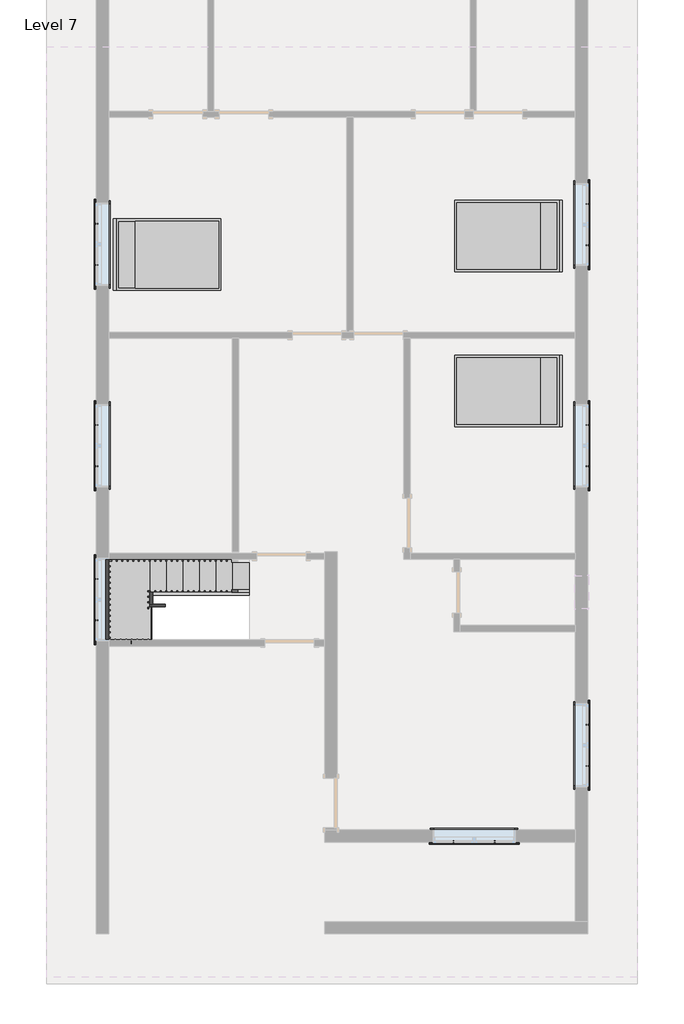
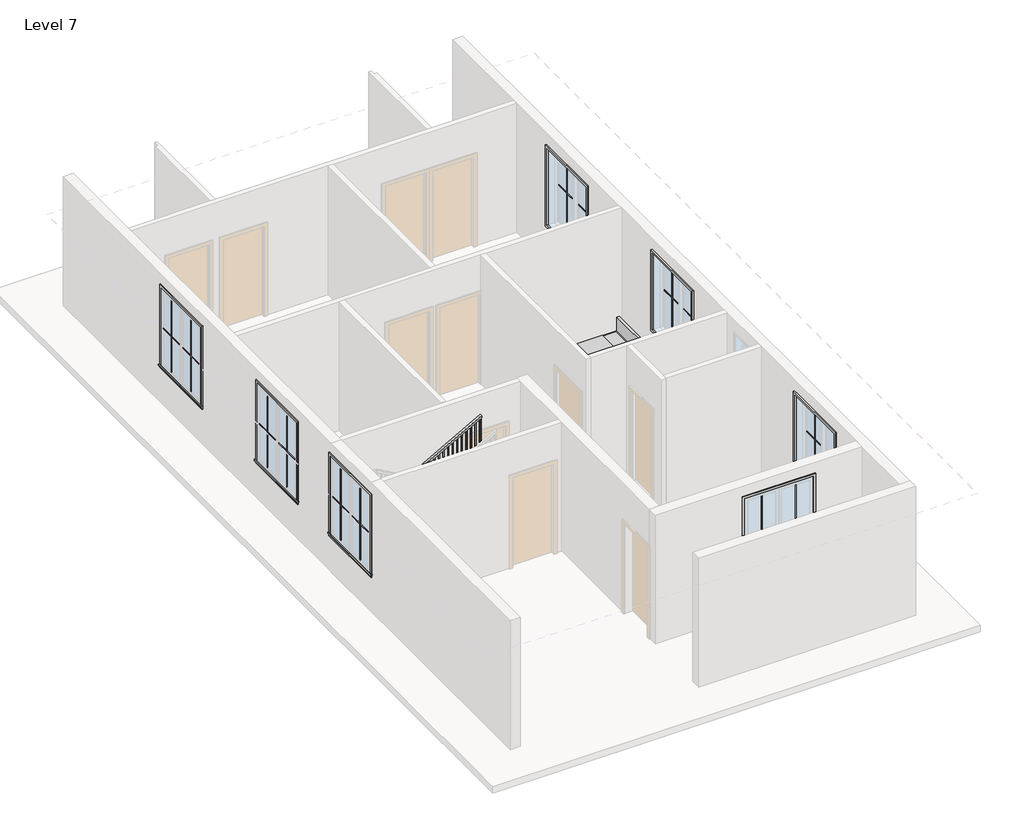
# One storey, part 3 of 3: 28 proxies, 6 members, 3 furniture elements, 1 railing, 1 stair flight.
"""IFC4 building model written with IfcOpenShell, lengths in millimetres."""

from ifc_helpers import new_model, si_unit, frame, origin, place, context, project, spatial, polyline, outline, extrude, faceted_brep, transform, mapped, element, save
from components import muntin_pattern_2x2_muntin_pattern_2x2_f6a80940, muntin_pattern_2x2_muntin_pattern_2x2_09b00a1c, trim_window_exterior_flat_with_sill_698ed857, trim_window_interior_flat_picture_frame_92551a5e, bed_17739_bed_17739_15c61121, stair_flight_6e983af9

model = new_model("IFC4")

# Units and contexts
model_context = context("Model", 3, world=origin())
ifc_project = project(units=[si_unit("LENGTHUNIT", "METRE", prefix="MILLI")], contexts=[model_context])

# Site, building, storey
site = spatial("IfcSite", under=ifc_project)
building = spatial("IfcBuilding", under=site)
storey = spatial("IfcBuildingStorey", under=building, Name="Level 7", Elevation=16002.0)

# Proxies
placement = place(None, origin())
muntin_pattern_2x2_muntin_pattern_2x2_shape = muntin_pattern_2x2_muntin_pattern_2x2_f6a80940(model_context)
element("IfcBuildingElementProxy", 1, Name="Muntin Pattern_2x2 : Muntin Pattern_2x2", ObjectType="Muntin Pattern_2x2 : Muntin Pattern_2x2", at=placement, inside=storey, context=model_context, shape_type="MappedRepresentation", body=[
    mapped(muntin_pattern_2x2_muntin_pattern_2x2_shape, transform((-5778.6870155, 3260.8309309, 16986.25), x_axis=(0.0, 1.0, 0.0), y_axis=(-1.0, 0.0, 0.0), z_axis=(0.0, 0.0, 1.0))),
])
element("IfcBuildingElementProxy", 2, Name="Muntin Pattern_2x2 : Muntin Pattern_2x2", ObjectType="Muntin Pattern_2x2 : Muntin Pattern_2x2", at=placement, inside=storey, context=model_context, shape_type="MappedRepresentation", body=[
    mapped(muntin_pattern_2x2_muntin_pattern_2x2_shape, transform((3270.0629845, 4381.6059309, 16986.25), x_axis=(0.0, -1.0, 0.0), y_axis=(1.0, 0.0, 0.0), z_axis=(0.0, 0.0, 1.0))),
])
element("IfcBuildingElementProxy", 3, Name="Muntin Pattern_2x2 : Muntin Pattern_2x2", ObjectType="Muntin Pattern_2x2 : Muntin Pattern_2x2", at=placement, inside=storey, context=model_context, shape_type="MappedRepresentation", body=[
    mapped(muntin_pattern_2x2_muntin_pattern_2x2_shape, transform((3270.0629845, 304.9059309, 16986.25), x_axis=(0.0, -1.0, 0.0), y_axis=(1.0, 0.0, 0.0), z_axis=(0.0, 0.0, 1.0))),
])
element("IfcBuildingElementProxy", 4, Name="Muntin Pattern_2x2 : Muntin Pattern_2x2", ObjectType="Muntin Pattern_2x2 : Muntin Pattern_2x2", at=placement, inside=storey, context=model_context, shape_type="MappedRepresentation", body=[
    mapped(muntin_pattern_2x2_muntin_pattern_2x2_shape, transform((3270.0629845, -5219.5940691, 16986.25), x_axis=(0.0, -1.0, 0.0), y_axis=(1.0, 0.0, 0.0), z_axis=(0.0, 0.0, 1.0))),
])
element("IfcBuildingElementProxy", 5, Name="Muntin Pattern_2x2 : Muntin Pattern_2x2", ObjectType="Muntin Pattern_2x2 : Muntin Pattern_2x2", at=placement, inside=storey, context=model_context, shape_type="MappedRepresentation", body=[
    mapped(muntin_pattern_2x2_muntin_pattern_2x2_shape, transform((1563.5004845, -7380.1815691, 16986.25), x_axis=(-1.0, 0.0, 0.0), y_axis=(0.0, -1.0, 0.0), z_axis=(0.0, 0.0, 1.0))),
])
element("IfcBuildingElementProxy", 6, Name="Muntin Pattern_2x2 : Muntin Pattern_2x2", ObjectType="Muntin Pattern_2x2 : Muntin Pattern_2x2", at=placement, inside=storey, context=model_context, shape_type="MappedRepresentation", body=[
    mapped(muntin_pattern_2x2_muntin_pattern_2x2_shape, transform((-5778.6870155, -3292.3690691, 16986.25), x_axis=(0.0, 1.0, 0.0), y_axis=(-1.0, 0.0, 0.0), z_axis=(0.0, 0.0, 1.0))),
])
element("IfcBuildingElementProxy", 7, Name="Muntin Pattern_2x2 : Muntin Pattern_2x2", ObjectType="Muntin Pattern_2x2 : Muntin Pattern_2x2", at=placement, inside=storey, context=model_context, shape_type="MappedRepresentation", body=[
    mapped(muntin_pattern_2x2_muntin_pattern_2x2_shape, transform((-5778.6870155, -453.9190691, 16986.25), x_axis=(0.0, 1.0, 0.0), y_axis=(-1.0, 0.0, 0.0), z_axis=(0.0, 0.0, 1.0))),
])
muntin_pattern_2x2_muntin_pattern_2x2_2_shape = muntin_pattern_2x2_muntin_pattern_2x2_09b00a1c(model_context)
element("IfcBuildingElementProxy", 8, Name="Muntin Pattern_2x2 : Muntin Pattern_2x2", ObjectType="Muntin Pattern_2x2 : Muntin Pattern_2x2", at=placement, inside=storey, context=model_context, shape_type="MappedRepresentation", body=[
    mapped(muntin_pattern_2x2_muntin_pattern_2x2_2_shape, transform((-5778.6870155, 4019.6559309, 16986.25), x_axis=(0.0, -1.0, 0.0), y_axis=(1.0, 0.0, 0.0), z_axis=(0.0, 0.0, 1.0))),
])
element("IfcBuildingElementProxy", 9, Name="Muntin Pattern_2x2 : Muntin Pattern_2x2", ObjectType="Muntin Pattern_2x2 : Muntin Pattern_2x2", at=placement, inside=storey, context=model_context, shape_type="MappedRepresentation", body=[
    mapped(muntin_pattern_2x2_muntin_pattern_2x2_2_shape, transform((3270.0629845, 3622.7809309, 16986.25), x_axis=(0.0, 1.0, 0.0), y_axis=(-1.0, 0.0, 0.0), z_axis=(0.0, 0.0, 1.0))),
])
element("IfcBuildingElementProxy", 10, Name="Muntin Pattern_2x2 : Muntin Pattern_2x2", ObjectType="Muntin Pattern_2x2 : Muntin Pattern_2x2", at=placement, inside=storey, context=model_context, shape_type="MappedRepresentation", body=[
    mapped(muntin_pattern_2x2_muntin_pattern_2x2_2_shape, transform((3270.0629845, -453.9190691, 16986.25), x_axis=(0.0, 1.0, 0.0), y_axis=(-1.0, 0.0, 0.0), z_axis=(0.0, 0.0, 1.0))),
])
element("IfcBuildingElementProxy", 11, Name="Muntin Pattern_2x2 : Muntin Pattern_2x2", ObjectType="Muntin Pattern_2x2 : Muntin Pattern_2x2", at=placement, inside=storey, context=model_context, shape_type="MappedRepresentation", body=[
    mapped(muntin_pattern_2x2_muntin_pattern_2x2_2_shape, transform((3270.0629845, -5978.4190691, 16986.25), x_axis=(0.0, 1.0, 0.0), y_axis=(-1.0, 0.0, 0.0), z_axis=(0.0, 0.0, 1.0))),
])
element("IfcBuildingElementProxy", 12, Name="Muntin Pattern_2x2 : Muntin Pattern_2x2", ObjectType="Muntin Pattern_2x2 : Muntin Pattern_2x2", at=placement, inside=storey, context=model_context, shape_type="MappedRepresentation", body=[
    mapped(muntin_pattern_2x2_muntin_pattern_2x2_2_shape, transform((804.6754845, -7380.1815691, 16986.25), x_axis=(1.0, 0.0, 0.0), y_axis=(0.0, 1.0, 0.0), z_axis=(0.0, 0.0, 1.0))),
])
element("IfcBuildingElementProxy", 13, Name="Muntin Pattern_2x2 : Muntin Pattern_2x2", ObjectType="Muntin Pattern_2x2 : Muntin Pattern_2x2", at=placement, inside=storey, context=model_context, shape_type="MappedRepresentation", body=[
    mapped(muntin_pattern_2x2_muntin_pattern_2x2_2_shape, transform((-5778.6870155, -2533.5440691, 16986.25), x_axis=(0.0, -1.0, 0.0), y_axis=(1.0, 0.0, 0.0), z_axis=(0.0, 0.0, 1.0))),
])
element("IfcBuildingElementProxy", 14, Name="Muntin Pattern_2x2 : Muntin Pattern_2x2", ObjectType="Muntin Pattern_2x2 : Muntin Pattern_2x2", at=placement, inside=storey, context=model_context, shape_type="MappedRepresentation", body=[
    mapped(muntin_pattern_2x2_muntin_pattern_2x2_2_shape, transform((-5778.6870155, 304.9059309, 16986.25), x_axis=(0.0, -1.0, 0.0), y_axis=(1.0, 0.0, 0.0), z_axis=(0.0, 0.0, 1.0))),
])
trim_window_exterior_flat_with_sill_shape = trim_window_exterior_flat_with_sill_698ed857(model_context)
element("IfcBuildingElementProxy", 15, Name="Trim-Window-Exterior-Flat : with Sill", ObjectType="Trim-Window-Exterior-Flat : with Sill", at=placement, inside=storey, context=model_context, shape_type="MappedRepresentation", body=[
    mapped(trim_window_exterior_flat_with_sill_shape, transform((-5788.2120155, 3640.2434309, 18745.2), x_axis=(0.0, -1.0, 0.0), y_axis=(0.0, 0.0, 1.0), z_axis=(-1.0, 0.0, 0.0))),
])
element("IfcBuildingElementProxy", 16, Name="Trim-Window-Exterior-Flat : with Sill", ObjectType="Trim-Window-Exterior-Flat : with Sill", at=placement, inside=storey, context=model_context, shape_type="MappedRepresentation", body=[
    mapped(trim_window_exterior_flat_with_sill_shape, transform((3279.5879845, 4002.1934309, 18745.2), x_axis=(0.0, 1.0, 0.0), y_axis=(0.0, 0.0, 1.0), z_axis=(1.0, 0.0, 0.0))),
])
element("IfcBuildingElementProxy", 17, Name="Trim-Window-Exterior-Flat : with Sill", ObjectType="Trim-Window-Exterior-Flat : with Sill", at=placement, inside=storey, context=model_context, shape_type="MappedRepresentation", body=[
    mapped(trim_window_exterior_flat_with_sill_shape, transform((3279.5879845, -74.5065691, 18745.2), x_axis=(0.0, 1.0, 0.0), y_axis=(0.0, 0.0, 1.0), z_axis=(1.0, 0.0, 0.0))),
])
element("IfcBuildingElementProxy", 18, Name="Trim-Window-Exterior-Flat : with Sill", ObjectType="Trim-Window-Exterior-Flat : with Sill", at=placement, inside=storey, context=model_context, shape_type="MappedRepresentation", body=[
    mapped(trim_window_exterior_flat_with_sill_shape, transform((3279.5879845, -5599.0065691, 18745.2), x_axis=(0.0, 1.0, 0.0), y_axis=(0.0, 0.0, 1.0), z_axis=(1.0, 0.0, 0.0))),
])
element("IfcBuildingElementProxy", 19, Name="Trim-Window-Exterior-Flat : with Sill", ObjectType="Trim-Window-Exterior-Flat : with Sill", at=placement, inside=storey, context=model_context, shape_type="MappedRepresentation", body=[
    mapped(trim_window_exterior_flat_with_sill_shape, transform((1184.0879845, -7389.7065691, 18745.2), x_axis=(1.0, 0.0, 0.0), y_axis=(0.0, 0.0, 1.0), z_axis=(0.0, -1.0, 0.0))),
])
element("IfcBuildingElementProxy", 20, Name="Trim-Window-Exterior-Flat : with Sill", ObjectType="Trim-Window-Exterior-Flat : with Sill", at=placement, inside=storey, context=model_context, shape_type="MappedRepresentation", body=[
    mapped(trim_window_exterior_flat_with_sill_shape, transform((-5788.2120155, -2912.9565691, 18745.2), x_axis=(0.0, -1.0, 0.0), y_axis=(0.0, 0.0, 1.0), z_axis=(-1.0, 0.0, 0.0))),
])
element("IfcBuildingElementProxy", 21, Name="Trim-Window-Exterior-Flat : with Sill", ObjectType="Trim-Window-Exterior-Flat : with Sill", at=placement, inside=storey, context=model_context, shape_type="MappedRepresentation", body=[
    mapped(trim_window_exterior_flat_with_sill_shape, transform((-5788.2120155, -74.5065691, 18745.2), x_axis=(0.0, -1.0, 0.0), y_axis=(0.0, 0.0, 1.0), z_axis=(-1.0, 0.0, 0.0))),
])
trim_window_interior_flat_picture_frame_shape = trim_window_interior_flat_picture_frame_92551a5e(model_context)
element("IfcBuildingElementProxy", 22, Name="Trim-Window-Interior-Flat : Picture Frame", ObjectType="Trim-Window-Interior-Flat : Picture Frame", at=placement, inside=storey, context=model_context, shape_type="MappedRepresentation", body=[
    mapped(trim_window_interior_flat_picture_frame_shape, transform((-5559.6120155, 3640.2434309, 18745.2), x_axis=(0.0, 1.0, 0.0), y_axis=(0.0, 0.0, 1.0), z_axis=(1.0, 0.0, 0.0))),
])
element("IfcBuildingElementProxy", 23, Name="Trim-Window-Interior-Flat : Picture Frame", ObjectType="Trim-Window-Interior-Flat : Picture Frame", at=placement, inside=storey, context=model_context, shape_type="MappedRepresentation", body=[
    mapped(trim_window_interior_flat_picture_frame_shape, transform((3050.9879845, 4002.1934309, 18745.2), x_axis=(0.0, -1.0, 0.0), y_axis=(0.0, 0.0, 1.0), z_axis=(-1.0, 0.0, 0.0))),
])
element("IfcBuildingElementProxy", 24, Name="Trim-Window-Interior-Flat : Picture Frame", ObjectType="Trim-Window-Interior-Flat : Picture Frame", at=placement, inside=storey, context=model_context, shape_type="MappedRepresentation", body=[
    mapped(trim_window_interior_flat_picture_frame_shape, transform((3050.9879845, -74.5065691, 18745.2), x_axis=(0.0, -1.0, 0.0), y_axis=(0.0, 0.0, 1.0), z_axis=(-1.0, 0.0, 0.0))),
])
element("IfcBuildingElementProxy", 25, Name="Trim-Window-Interior-Flat : Picture Frame", ObjectType="Trim-Window-Interior-Flat : Picture Frame", at=placement, inside=storey, context=model_context, shape_type="MappedRepresentation", body=[
    mapped(trim_window_interior_flat_picture_frame_shape, transform((3050.9879845, -5599.0065691, 18745.2), x_axis=(0.0, -1.0, 0.0), y_axis=(0.0, 0.0, 1.0), z_axis=(-1.0, 0.0, 0.0))),
])
element("IfcBuildingElementProxy", 26, Name="Trim-Window-Interior-Flat : Picture Frame", ObjectType="Trim-Window-Interior-Flat : Picture Frame", at=placement, inside=storey, context=model_context, shape_type="MappedRepresentation", body=[
    mapped(trim_window_interior_flat_picture_frame_shape, transform((1184.0879845, -7161.1065691, 18745.2), x_axis=(-1.0, 0.0, 0.0), y_axis=(0.0, 0.0, 1.0), z_axis=(0.0, 1.0, 0.0))),
])
element("IfcBuildingElementProxy", 27, Name="Trim-Window-Interior-Flat : Picture Frame", ObjectType="Trim-Window-Interior-Flat : Picture Frame", at=placement, inside=storey, context=model_context, shape_type="MappedRepresentation", body=[
    mapped(trim_window_interior_flat_picture_frame_shape, transform((-5559.6120155, -2912.9565691, 18745.2), x_axis=(0.0, 1.0, 0.0), y_axis=(0.0, 0.0, 1.0), z_axis=(1.0, 0.0, 0.0))),
])
element("IfcBuildingElementProxy", 28, Name="Trim-Window-Interior-Flat : Picture Frame", ObjectType="Trim-Window-Interior-Flat : Picture Frame", at=placement, inside=storey, context=model_context, shape_type="MappedRepresentation", body=[
    mapped(trim_window_interior_flat_picture_frame_shape, transform((-5559.6120155, -74.5065691, 18745.2), x_axis=(0.0, 1.0, 0.0), y_axis=(0.0, 0.0, 1.0), z_axis=(1.0, 0.0, 0.0))),
])

# Furniture
bed_17739_bed_17739_shape = bed_17739_bed_17739_15c61121(model_context)
element("IfcFurniture", 29, ObjectType="Bed_17739 : Bed_17739", at=placement, inside=storey, context=model_context, shape_type="MappedRepresentation", body=[
    mapped(bed_17739_bed_17739_shape, transform((-4454.7120155, 3449.7434309, 16002.0), x_axis=(0.0, 1.0, 0.0), y_axis=(-1.0, 0.0, 0.0), z_axis=(0.0, 0.0, 1.0))),
])
element("IfcFurniture", 30, ObjectType="Bed_17739 : Bed_17739", at=placement, inside=storey, context=model_context, shape_type="MappedRepresentation", body=[
    mapped(bed_17739_bed_17739_shape, transform((1793.6879845, 3792.6434309, 16002.0), x_axis=(0.0, -1.0, 0.0), y_axis=(1.0, 0.0, 0.0), z_axis=(0.0, 0.0, 1.0))),
])
element("IfcFurniture", 31, ObjectType="Bed_17739 : Bed_17739", at=placement, inside=storey, context=model_context, shape_type="MappedRepresentation", body=[
    mapped(bed_17739_bed_17739_shape, transform((1793.6879845, 935.1434309, 16002.0), x_axis=(0.0, -1.0, 0.0), y_axis=(1.0, 0.0, 0.0), z_axis=(0.0, 0.0, 1.0))),
])

# Members
element("IfcMember", 32, ObjectType="Stringer - 2\" Width", at=placement, inside=storey, context=model_context, shape_type="SweptSolid", body=[
    extrude(outline(polyline([(16002.0, -2968.8120155), (16209.5983948, -2968.8120155), (17197.3761726, -4746.8120155), (16848.6974984, -4746.8120155), (16002.0, -3222.7565183), (16002.0, -2968.8120155)])), frame((0.0, -2830.4065691, 0.0), z_axis=(0.0, 1.0, 0.0), x_axis=(0.0, 0.0, 1.0)), (0.0, 0.0, 1.0), 50.8),
])
element("IfcMember", 33, ObjectType="Stringer - 2\" Width", at=placement, inside=storey, context=model_context, shape_type="SweptSolid", body=[
    extrude(outline(polyline([(-4797.6120155, -2779.6065691), (-4746.8120155, -2779.6065691), (-4746.8120155, -2995.5065691), (-4797.6120155, -2995.5065691), (-4797.6120155, -2779.6065691)])), frame((0.0, 0.0, 16958.7333333), z_axis=(0.0, 0.0, 1.0), x_axis=(1.0, 0.0, 0.0)), (0.0, 0.0, 1.0), 304.8),
])
element("IfcMember", 34, ObjectType="Stringer - 2\" Width", at=placement, inside=storey, context=model_context, shape_type="SweptSolid", body=[
    extrude(outline(polyline([(17394.9317281, -4797.6120155), (17046.253054, -4797.6120155), (18062.253054, -2968.8120155), (18410.9317281, -2968.8120155), (17394.9317281, -4797.6120155)])), frame((0.0, -3046.3065691, 0.0), z_axis=(0.0, 1.0, 0.0), x_axis=(0.0, 0.0, 1.0)), (0.0, 0.0, 1.0), 50.8),
])
element("IfcMember", 35, ObjectType="Stringer - 2\" Width", at=placement, inside=storey, context=model_context, shape_type="SweptSolid", body=[
    extrude(outline(polyline([(16002.0, -2968.8120155), (16209.5983948, -2968.8120155), (17263.5333333, -4865.8949049), (17263.5333333, -5493.5165183), (16002.0, -3222.7565183), (16002.0, -2968.8120155)])), frame((0.0, -2170.0065691, 0.0), z_axis=(0.0, 1.0, 0.0), x_axis=(0.0, 0.0, 1.0)), (0.0, 0.0, 1.0), 50.8),
])
element("IfcMember", 36, ObjectType="Stringer - 2\" Width", at=placement, inside=storey, context=model_context, shape_type="SweptSolid", body=[
    extrude(outline(polyline([(-5610.4120155, -2119.2065691), (-5559.6120155, -2119.2065691), (-5559.6120155, -3674.9565691), (-5610.4120155, -3674.9565691), (-5610.4120155, -2119.2065691)])), frame((0.0, 0.0, 16958.7333333), z_axis=(0.0, 0.0, 1.0), x_axis=(1.0, 0.0, 0.0)), (0.0, 0.0, 1.0), 304.8),
])
element("IfcMember", 37, ObjectType="Stringer - 2\" Width", at=placement, inside=storey, context=model_context, shape_type="SweptSolid", body=[
    extrude(outline(polyline([(16958.7333333, -4955.1475127), (18062.253054, -2968.8120155), (18410.9317281, -2968.8120155), (16958.7333333, -5582.7691261), (16958.7333333, -4955.1475127)])), frame((0.0, -3725.7565691, 0.0), z_axis=(0.0, 1.0, 0.0), x_axis=(0.0, 0.0, 1.0)), (0.0, 0.0, 1.0), 50.8),
])

# Railing
element("IfcRailing", 38, ObjectType="Handrail - Rectangular", at=placement, inside=storey, context=model_context, shape_type="SolidModel", body=[
    faceted_brep([(-2968.8120155, -2779.6065691, 17085.7333333), (-2968.8120155, -2779.6065691, 17027.620221), (-2968.8120155, -2728.8065691, 17027.620221), (-2968.8120155, -2728.8065691, 17085.7333333), (-4721.4120155, -2779.6065691, 18059.4), (-4772.2120155, -2779.6065691, 18029.5091099), (-4772.2120155, -2728.8065691, 18029.5091099), (-4721.4120155, -2728.8065691, 18059.4), (-4721.4120155, -2779.6065691, 18101.7333333), (-4772.2120155, -2779.6065691, 18050.9333333), (-4772.2120155, -2728.8065691, 18050.9333333), (-4721.4120155, -2728.8065691, 18101.7333333), (-4797.6120155, -2779.6065691, 18101.7333333), (-4797.6120155, -2779.6065691, 18050.9333333), (-4848.4120155, -2728.8065691, 18050.9333333), (-4848.4120155, -2728.8065691, 18101.7333333), (-4797.6120155, -2855.8065691, 18101.7333333), (-4797.6120155, -2855.8065691, 18050.9333333), (-4848.4120155, -2855.8065691, 18050.9333333), (-4848.4120155, -2855.8065691, 18101.7333333), (-4797.6120155, -2970.1065691, 18101.7333333), (-4797.6120155, -3020.9065691, 18050.9333333), (-4848.4120155, -3020.9065691, 18050.9333333), (-4848.4120155, -2970.1065691, 18101.7333333), (-4797.6120155, -2970.1065691, 18313.4), (-4797.6120155, -3020.9065691, 18262.6), (-4848.4120155, -3020.9065691, 18262.6), (-4848.4120155, -2970.1065691, 18313.4), (-4797.6120155, -3046.3065691, 18313.4), (-4797.6120155, -3046.3065691, 18262.6), (-4848.4120155, -3097.1065691, 18262.6), (-4848.4120155, -3097.1065691, 18313.4), (-4721.4120155, -3046.3065691, 18313.4), (-4708.2484132, -3046.3065691, 18262.6), (-4708.2484132, -3097.1065691, 18262.6), (-4721.4120155, -3097.1065691, 18313.4), (-2968.8120155, -3046.3065691, 19287.0666667), (-2968.8120155, -3097.1065691, 19287.0666667), (-2968.8120155, -3097.1065691, 19228.9535543), (-2968.8120155, -3046.3065691, 19228.9535543)], [[[0, 1, 2, 3]], [[1, 0, 4, 5]], [[2, 1, 5, 6]], [[3, 2, 6, 7]], [[0, 3, 7, 4]], [[5, 4, 8, 9]], [[6, 5, 9, 10]], [[7, 6, 10, 11]], [[4, 7, 11, 8]], [[9, 8, 12, 13]], [[10, 9, 13, 14]], [[11, 10, 14, 15]], [[8, 11, 15, 12]], [[13, 12, 16, 17]], [[14, 13, 17, 18]], [[15, 14, 18, 19]], [[12, 15, 19, 16]], [[17, 16, 20, 21]], [[18, 17, 21, 22]], [[19, 18, 22, 23]], [[16, 19, 23, 20]], [[21, 20, 24, 25]], [[22, 21, 25, 26]], [[23, 22, 26, 27]], [[20, 23, 27, 24]], [[25, 24, 28, 29]], [[26, 25, 29, 30]], [[27, 26, 30, 31]], [[24, 27, 31, 28]], [[29, 28, 32, 33]], [[30, 29, 33, 34]], [[31, 30, 34, 35]], [[28, 31, 35, 32]], [[36, 37, 38, 39]], [[33, 32, 36, 39]], [[34, 33, 39, 38]], [[35, 34, 38, 37]], [[32, 35, 37, 36]]]),
    extrude(outline(polyline([(19209.5507765, -3003.7370155), (18203.3333333, -3003.7370155), (18203.3333333, -2984.6870155), (19220.1341099, -2984.6870155), (19209.5507765, -3003.7370155)])), frame((0.0, -3081.2315691, 0.0), z_axis=(0.0, 1.0, 0.0), x_axis=(0.0, 0.0, 1.0)), (0.0, 0.0, 1.0), 19.05),
    extrude(outline(polyline([(19153.1063321, -3105.3370155), (18203.3333333, -3105.3370155), (18203.3333333, -3086.2870155), (19163.6896654, -3086.2870155), (19153.1063321, -3105.3370155)])), frame((0.0, -3081.2315691, 0.0), z_axis=(0.0, 1.0, 0.0), x_axis=(0.0, 0.0, 1.0)), (0.0, 0.0, 1.0), 19.05),
    extrude(outline(polyline([(19096.6618876, -3206.9370155), (18203.3333333, -3206.9370155), (18203.3333333, -3187.8870155), (19107.245221, -3187.8870155), (19096.6618876, -3206.9370155)])), frame((0.0, -3081.2315691, 0.0), z_axis=(0.0, 1.0, 0.0), x_axis=(0.0, 0.0, 1.0)), (0.0, 0.0, 1.0), 19.05),
    extrude(outline(polyline([(19040.2174432, -3308.5370155), (18034.0, -3308.5370155), (18034.0, -3289.4870155), (19050.8007765, -3289.4870155), (19040.2174432, -3308.5370155)])), frame((0.0, -3081.2315691, 0.0), z_axis=(0.0, 1.0, 0.0), x_axis=(0.0, 0.0, 1.0)), (0.0, 0.0, 1.0), 19.05),
    extrude(outline(polyline([(18983.7729988, -3410.1370155), (18034.0, -3410.1370155), (18034.0, -3391.0870155), (18994.3563321, -3391.0870155), (18983.7729988, -3410.1370155)])), frame((0.0, -3081.2315691, 0.0), z_axis=(0.0, 1.0, 0.0), x_axis=(0.0, 0.0, 1.0)), (0.0, 0.0, 1.0), 19.05),
    extrude(outline(polyline([(18927.3285543, -3511.7370155), (18034.0, -3511.7370155), (18034.0, -3492.6870155), (18937.9118876, -3492.6870155), (18927.3285543, -3511.7370155)])), frame((0.0, -3081.2315691, 0.0), z_axis=(0.0, 1.0, 0.0), x_axis=(0.0, 0.0, 1.0)), (0.0, 0.0, 1.0), 19.05),
    extrude(outline(polyline([(18870.8841099, -3613.3370155), (17864.6666667, -3613.3370155), (17864.6666667, -3594.2870155), (18881.4674432, -3594.2870155), (18870.8841099, -3613.3370155)])), frame((0.0, -3081.2315691, 0.0), z_axis=(0.0, 1.0, 0.0), x_axis=(0.0, 0.0, 1.0)), (0.0, 0.0, 1.0), 19.05),
    extrude(outline(polyline([(18814.4396654, -3714.9370155), (17864.6666667, -3714.9370155), (17864.6666667, -3695.8870155), (18825.0229988, -3695.8870155), (18814.4396654, -3714.9370155)])), frame((0.0, -3081.2315691, 0.0), z_axis=(0.0, 1.0, 0.0), x_axis=(0.0, 0.0, 1.0)), (0.0, 0.0, 1.0), 19.05),
    extrude(outline(polyline([(18757.995221, -3816.5370155), (17864.6666667, -3816.5370155), (17864.6666667, -3797.4870155), (18768.5785543, -3797.4870155), (18757.995221, -3816.5370155)])), frame((0.0, -3081.2315691, 0.0), z_axis=(0.0, 1.0, 0.0), x_axis=(0.0, 0.0, 1.0)), (0.0, 0.0, 1.0), 19.05),
    extrude(outline(polyline([(18701.5507765, -3918.1370155), (17695.3333333, -3918.1370155), (17695.3333333, -3899.0870155), (18712.1341099, -3899.0870155), (18701.5507765, -3918.1370155)])), frame((0.0, -3081.2315691, 0.0), z_axis=(0.0, 1.0, 0.0), x_axis=(0.0, 0.0, 1.0)), (0.0, 0.0, 1.0), 19.05),
    extrude(outline(polyline([(18645.1063321, -4019.7370155), (17695.3333333, -4019.7370155), (17695.3333333, -4000.6870155), (18655.6896654, -4000.6870155), (18645.1063321, -4019.7370155)])), frame((0.0, -3081.2315691, 0.0), z_axis=(0.0, 1.0, 0.0), x_axis=(0.0, 0.0, 1.0)), (0.0, 0.0, 1.0), 19.05),
    extrude(outline(polyline([(18588.6618876, -4121.3370155), (17695.3333333, -4121.3370155), (17695.3333333, -4102.2870155), (18599.245221, -4102.2870155), (18588.6618876, -4121.3370155)])), frame((0.0, -3081.2315691, 0.0), z_axis=(0.0, 1.0, 0.0), x_axis=(0.0, 0.0, 1.0)), (0.0, 0.0, 1.0), 19.05),
    extrude(outline(polyline([(18532.2174432, -4222.9370155), (17526.0, -4222.9370155), (17526.0, -4203.8870155), (18542.8007765, -4203.8870155), (18532.2174432, -4222.9370155)])), frame((0.0, -3081.2315691, 0.0), z_axis=(0.0, 1.0, 0.0), x_axis=(0.0, 0.0, 1.0)), (0.0, 0.0, 1.0), 19.05),
    extrude(outline(polyline([(18475.7729988, -4324.5370155), (17526.0, -4324.5370155), (17526.0, -4305.4870155), (18486.3563321, -4305.4870155), (18475.7729988, -4324.5370155)])), frame((0.0, -3081.2315691, 0.0), z_axis=(0.0, 1.0, 0.0), x_axis=(0.0, 0.0, 1.0)), (0.0, 0.0, 1.0), 19.05),
    extrude(outline(polyline([(18419.3285543, -4426.1370155), (17526.0, -4426.1370155), (17526.0, -4407.0870155), (18429.9118876, -4407.0870155), (18419.3285543, -4426.1370155)])), frame((0.0, -3081.2315691, 0.0), z_axis=(0.0, 1.0, 0.0), x_axis=(0.0, 0.0, 1.0)), (0.0, 0.0, 1.0), 19.05),
    extrude(outline(polyline([(18362.8841099, -4527.7370155), (17356.6666667, -4527.7370155), (17356.6666667, -4508.6870155), (18373.4674432, -4508.6870155), (18362.8841099, -4527.7370155)])), frame((0.0, -3081.2315691, 0.0), z_axis=(0.0, 1.0, 0.0), x_axis=(0.0, 0.0, 1.0)), (0.0, 0.0, 1.0), 19.05),
    extrude(outline(polyline([(18306.4396654, -4629.3370155), (17356.6666667, -4629.3370155), (17356.6666667, -4610.2870155), (18317.0229988, -4610.2870155), (18306.4396654, -4629.3370155)])), frame((0.0, -3081.2315691, 0.0), z_axis=(0.0, 1.0, 0.0), x_axis=(0.0, 0.0, 1.0)), (0.0, 0.0, 1.0), 19.05),
    extrude(outline(polyline([(18249.995221, -4730.9370155), (17356.6666667, -4730.9370155), (17356.6666667, -4711.8870155), (18260.5785543, -4711.8870155), (18249.995221, -4730.9370155)])), frame((0.0, -3081.2315691, 0.0), z_axis=(0.0, 1.0, 0.0), x_axis=(0.0, 0.0, 1.0)), (0.0, 0.0, 1.0), 19.05),
    extrude(outline(polyline([(-4813.4870155, -3049.4815691), (-4813.4870155, -3068.5315691), (-4832.5370155, -3068.5315691), (-4832.5370155, -3049.4815691), (-4813.4870155, -3049.4815691)])), frame((0.0, 0.0, 17187.3333333), z_axis=(0.0, 0.0, 1.0), x_axis=(1.0, 0.0, 0.0)), (0.0, 0.0, 1.0), 1075.2666667),
    extrude(outline(polyline([(-4813.4870155, -2947.8815691), (-4813.4870155, -2966.9315691), (-4832.5370155, -2966.9315691), (-4832.5370155, -2947.8815691), (-4813.4870155, -2947.8815691)])), frame((0.0, 0.0, 17187.3333333), z_axis=(0.0, 0.0, 1.0), x_axis=(1.0, 0.0, 0.0)), (0.0, 0.0, 1.0), 863.6),
    extrude(outline(polyline([(-4813.4870155, -2846.2815691), (-4813.4870155, -2865.3315691), (-4832.5370155, -2865.3315691), (-4832.5370155, -2846.2815691), (-4813.4870155, -2846.2815691)])), frame((0.0, 0.0, 17187.3333333), z_axis=(0.0, 0.0, 1.0), x_axis=(1.0, 0.0, 0.0)), (0.0, 0.0, 1.0), 863.6),
    extrude(outline(polyline([(-4788.0870155, -2763.7315691), (-4807.1370155, -2763.7315691), (-4807.1370155, -2744.6815691), (-4788.0870155, -2744.6815691), (-4788.0870155, -2763.7315691)])), frame((0.0, 0.0, 17187.3333333), z_axis=(0.0, 0.0, 1.0), x_axis=(1.0, 0.0, 0.0)), (0.0, 0.0, 1.0), 863.6),
    extrude(outline(polyline([(17992.4674432, -4705.5370155), (17018.0, -4705.5370155), (17018.0, -4686.4870155), (17981.8841099, -4686.4870155), (17992.4674432, -4705.5370155)])), frame((0.0, -2763.7315691, 0.0), z_axis=(0.0, 1.0, 0.0), x_axis=(0.0, 0.0, 1.0)), (0.0, 0.0, 1.0), 19.05),
    extrude(outline(polyline([(17936.0229988, -4603.9370155), (17018.0, -4603.9370155), (17018.0, -4584.8870155), (17925.4396654, -4584.8870155), (17936.0229988, -4603.9370155)])), frame((0.0, -2763.7315691, 0.0), z_axis=(0.0, 1.0, 0.0), x_axis=(0.0, 0.0, 1.0)), (0.0, 0.0, 1.0), 19.05),
    extrude(outline(polyline([(17879.5785543, -4502.3370155), (17018.0, -4502.3370155), (17018.0, -4483.2870155), (17868.995221, -4483.2870155), (17879.5785543, -4502.3370155)])), frame((0.0, -2763.7315691, 0.0), z_axis=(0.0, 1.0, 0.0), x_axis=(0.0, 0.0, 1.0)), (0.0, 0.0, 1.0), 19.05),
    extrude(outline(polyline([(17823.1341099, -4400.7370155), (16848.6666667, -4400.7370155), (16848.6666667, -4381.6870155), (17812.5507765, -4381.6870155), (17823.1341099, -4400.7370155)])), frame((0.0, -2763.7315691, 0.0), z_axis=(0.0, 1.0, 0.0), x_axis=(0.0, 0.0, 1.0)), (0.0, 0.0, 1.0), 19.05),
    extrude(outline(polyline([(17766.6896654, -4299.1370155), (16848.6666667, -4299.1370155), (16848.6666667, -4280.0870155), (17756.1063321, -4280.0870155), (17766.6896654, -4299.1370155)])), frame((0.0, -2763.7315691, 0.0), z_axis=(0.0, 1.0, 0.0), x_axis=(0.0, 0.0, 1.0)), (0.0, 0.0, 1.0), 19.05),
    extrude(outline(polyline([(17710.245221, -4197.5370155), (16848.6666667, -4197.5370155), (16848.6666667, -4178.4870155), (17699.6618876, -4178.4870155), (17710.245221, -4197.5370155)])), frame((0.0, -2763.7315691, 0.0), z_axis=(0.0, 1.0, 0.0), x_axis=(0.0, 0.0, 1.0)), (0.0, 0.0, 1.0), 19.05),
    extrude(outline(polyline([(17653.8007765, -4095.9370155), (16679.3333333, -4095.9370155), (16679.3333333, -4076.8870155), (17643.2174432, -4076.8870155), (17653.8007765, -4095.9370155)])), frame((0.0, -2763.7315691, 0.0), z_axis=(0.0, 1.0, 0.0), x_axis=(0.0, 0.0, 1.0)), (0.0, 0.0, 1.0), 19.05),
    extrude(outline(polyline([(17597.3563321, -3994.3370155), (16679.3333333, -3994.3370155), (16679.3333333, -3975.2870155), (17586.7729988, -3975.2870155), (17597.3563321, -3994.3370155)])), frame((0.0, -2763.7315691, 0.0), z_axis=(0.0, 1.0, 0.0), x_axis=(0.0, 0.0, 1.0)), (0.0, 0.0, 1.0), 19.05),
    extrude(outline(polyline([(17540.9118876, -3892.7370155), (16679.3333333, -3892.7370155), (16679.3333333, -3873.6870155), (17530.3285543, -3873.6870155), (17540.9118876, -3892.7370155)])), frame((0.0, -2763.7315691, 0.0), z_axis=(0.0, 1.0, 0.0), x_axis=(0.0, 0.0, 1.0)), (0.0, 0.0, 1.0), 19.05),
    extrude(outline(polyline([(17484.4674432, -3791.1370155), (16510.0, -3791.1370155), (16510.0, -3772.0870155), (17473.8841099, -3772.0870155), (17484.4674432, -3791.1370155)])), frame((0.0, -2763.7315691, 0.0), z_axis=(0.0, 1.0, 0.0), x_axis=(0.0, 0.0, 1.0)), (0.0, 0.0, 1.0), 19.05),
    extrude(outline(polyline([(17428.0229988, -3689.5370155), (16510.0, -3689.5370155), (16510.0, -3670.4870155), (17417.4396654, -3670.4870155), (17428.0229988, -3689.5370155)])), frame((0.0, -2763.7315691, 0.0), z_axis=(0.0, 1.0, 0.0), x_axis=(0.0, 0.0, 1.0)), (0.0, 0.0, 1.0), 19.05),
    extrude(outline(polyline([(17371.5785543, -3587.9370155), (16510.0, -3587.9370155), (16510.0, -3568.8870155), (17360.995221, -3568.8870155), (17371.5785543, -3587.9370155)])), frame((0.0, -2763.7315691, 0.0), z_axis=(0.0, 1.0, 0.0), x_axis=(0.0, 0.0, 1.0)), (0.0, 0.0, 1.0), 19.05),
    extrude(outline(polyline([(17315.1341099, -3486.3370155), (16340.6666667, -3486.3370155), (16340.6666667, -3467.2870155), (17304.5507765, -3467.2870155), (17315.1341099, -3486.3370155)])), frame((0.0, -2763.7315691, 0.0), z_axis=(0.0, 1.0, 0.0), x_axis=(0.0, 0.0, 1.0)), (0.0, 0.0, 1.0), 19.05),
    extrude(outline(polyline([(17258.6896654, -3384.7370155), (16340.6666667, -3384.7370155), (16340.6666667, -3365.6870155), (17248.1063321, -3365.6870155), (17258.6896654, -3384.7370155)])), frame((0.0, -2763.7315691, 0.0), z_axis=(0.0, 1.0, 0.0), x_axis=(0.0, 0.0, 1.0)), (0.0, 0.0, 1.0), 19.05),
    extrude(outline(polyline([(17202.245221, -3283.1370155), (16340.6666667, -3283.1370155), (16340.6666667, -3264.0870155), (17191.6618876, -3264.0870155), (17202.245221, -3283.1370155)])), frame((0.0, -2763.7315691, 0.0), z_axis=(0.0, 1.0, 0.0), x_axis=(0.0, 0.0, 1.0)), (0.0, 0.0, 1.0), 19.05),
    extrude(outline(polyline([(17145.8007765, -3181.5370155), (16171.3333333, -3181.5370155), (16171.3333333, -3162.4870155), (17135.2174432, -3162.4870155), (17145.8007765, -3181.5370155)])), frame((0.0, -2763.7315691, 0.0), z_axis=(0.0, 1.0, 0.0), x_axis=(0.0, 0.0, 1.0)), (0.0, 0.0, 1.0), 19.05),
    extrude(outline(polyline([(17089.3563321, -3079.9370155), (16171.3333333, -3079.9370155), (16171.3333333, -3060.8870155), (17078.7729988, -3060.8870155), (17089.3563321, -3079.9370155)])), frame((0.0, -2763.7315691, 0.0), z_axis=(0.0, 1.0, 0.0), x_axis=(0.0, 0.0, 1.0)), (0.0, 0.0, 1.0), 19.05),
    extrude(outline(polyline([(-4813.4870155, -3062.1815691), (-4813.4870155, -3081.2315691), (-4832.5370155, -3081.2315691), (-4832.5370155, -3062.1815691), (-4813.4870155, -3062.1815691)])), frame((0.0, 0.0, 17187.3333333), z_axis=(0.0, 0.0, 1.0), x_axis=(1.0, 0.0, 0.0)), (0.0, 0.0, 1.0), 1075.2666667),
    extrude(outline(polyline([(-4813.4870155, -2763.7315691), (-4832.5370155, -2763.7315691), (-4832.5370155, -2744.6815691), (-4813.4870155, -2744.6815691), (-4813.4870155, -2763.7315691)])), frame((0.0, 0.0, 17187.3333333), z_axis=(0.0, 0.0, 1.0), x_axis=(1.0, 0.0, 0.0)), (0.0, 0.0, 1.0), 863.6),
    extrude(outline(polyline([(19218.370221, -2987.8620155), (18203.3333333, -2987.8620155), (18203.3333333, -2968.8120155), (19228.9535543, -2968.8120155), (19218.370221, -2987.8620155)])), frame((0.0, -3081.2315691, 0.0), z_axis=(0.0, 1.0, 0.0), x_axis=(0.0, 0.0, 1.0)), (0.0, 0.0, 1.0), 19.05),
    extrude(outline(polyline([(17038.2035543, -2987.8620155), (16171.3333333, -2987.8620155), (16171.3333333, -2968.8120155), (17027.620221, -2968.8120155), (17038.2035543, -2987.8620155)])), frame((0.0, -2763.7315691, 0.0), z_axis=(0.0, 1.0, 0.0), x_axis=(0.0, 0.0, 1.0)), (0.0, 0.0, 1.0), 19.05),
])

# Stair flight
stair_flight_shape = stair_flight_6e983af9(model_context)
element("IfcStairFlight", 39, ObjectType="2\" Tread 1\" Nosing 1/4\" Riser", at=placement, inside=storey, context=model_context, shape_type="MappedRepresentation", body=[
    mapped(stair_flight_shape, transform((0.0, 0.0, 0.0), x_axis=(1.0, 0.0, 0.0), y_axis=(0.0, 1.0, 0.0), z_axis=(0.0, 0.0, 1.0))),
])

save(model, "model.ifc")

# Revit data of these elements
# Type "Muntin Pattern_2x2 : Muntin Pattern_2x2"
#   Width [instance default] = 4' - 0"
#   Thickness = 0' - 0 1/2"
#   Height [instance default] = 4' - 0"
#   Distance = 0' - 0 3/4"
#   Interior Material [instance default] = none
#   Exterior Material [instance default] = none
#   Default Elevation = 0
# Type "Trim-Window-Exterior-Flat : with Sill"
#   Trim Width = 0' - 2 1/4"
#   Trim Thickness_Picture Frame = 0' - 1 1/4"
#   Trim Thickness_with Sill = 0' - 0 3/4"
#   Sill Thickness = 0' - 1 1/4"
#   Opening Width [instance default] = 2' - 0"
#   Opening Height [instance default] = 3' - 0"
#   Default Elevation = 4' - 0"
#   Sill = yes
#   Picture Frame = no
#   Trim Material [instance default] = none
# Type "Trim-Window-Interior-Flat : Picture Frame"
#   Trim Thickness_Picture Frame = 0' - 1 1/4"
#   Trim Width = 0' - 2 1/4"
#   Trim Thickness_with Sill = 0' - 0 3/4"
#   Sill Thickness = 0' - 1 1/4"
#   Opening Width [instance default] = 2' - 0"
#   Opening Height [instance default] = 3' - 0"
#   Default Elevation = 4' - 0"
#   Sill = no
#   Picture Frame = yes
#   Trim Material [instance default] = none
# Type "Bed_17739 : Bed_17739"
#   Default Elevation = 0
# Type "Handrail - Rectangular"
#   Assembly Code = "C2010400"
#   built-in parameter 1008612 = 0.0416667 (stored number, unit not read)
#   built-in parameter 1008611 = 0.0416667 (stored number, unit not read)
#   built-in parameter 1008609 = 0.333333 (stored number, unit not read)
#   built-in parameter 1008604 = 0.166667 (stored number, unit not read)
#   built-in parameter 1008603 = 0.166667 (stored number, unit not read)
#   Railing Height = 3' - 0"
#   built-in parameter 1008630 = 2
#   built-in parameter 1008610 = 2
#   built-in parameter 1008618 = Baluster - Square : 3/4"
# Elements 1, 2, 3, 4, 5, 6, 7, 8, 9, 10, 11, 12, 13, 14 (IfcBuildingElementProxy, "Muntin Pattern_2x2 : Muntin Pattern_2x2")
#   Width = 2' - 0 5/8"
#   Height = 5' - 6 1/2"
#   Interior Material = Wood - Stained
#   Exterior Material = Clad - White
#   Phase Created = New Construction
#   Materials on its faces: "Clad - White", "Wood - Stained"
# Elements 15, 16, 17, 18, 19, 20, 21 (IfcBuildingElementProxy, "Trim-Window-Exterior-Flat : with Sill")
#   Opening Width = 5' - 0"
#   Opening Height = 6' - 0"
#   Trim Material = Clad - White
#   Phase Created = New Construction
#   Materials on its faces: "Clad - White"
# Elements 22, 23, 24, 25, 26, 27, 28 (IfcBuildingElementProxy, "Trim-Window-Interior-Flat : Picture Frame")
#   Opening Width = 5' - 0"
#   Opening Height = 6' - 0"
#   Trim Material = Wood - Stained
#   Phase Created = New Construction
#   Materials on its faces: "Wood - Stained"
# Elements 29, 30, 31 (IfcFurniture, "Bed_17739 : Bed_17739")
#   Phase Created = New Construction
#   Materials on its faces: "legs", "sheets", "bed frame", "Blanket"
# Elements 32, 33, 34, 35, 36, 37 (IfcMember, "Stringer - 2\" Width")
#   Phase Created = New Construction
# Element 38 (IfcRailing, "Handrail - Rectangular")
#   Phase Created = New Construction
# Element 39 (IfcStairFlight, "2\" Tread 1\" Nosing 1/4\" Riser")
#   Phase Created = New Construction
# Materials
#   "Clad - White": class "Wood", colour RGB 242 242 238, transparency 0, Cost = 0
#   "Wood - Stained": class "Wood", colour RGB 224 178 126, transparency 0, Cost = 0
#   "legs": colour RGB 90 73 37, transparency 0, Cost = 0
#   "sheets": colour RGB 200 195 176, transparency 0, Cost = 0
#   "bed frame": colour RGB 90 73 37, transparency 0, Cost = 0
#   "Blanket": class "System", colour RGB 59 0 1, transparency 0, Cost = 0
